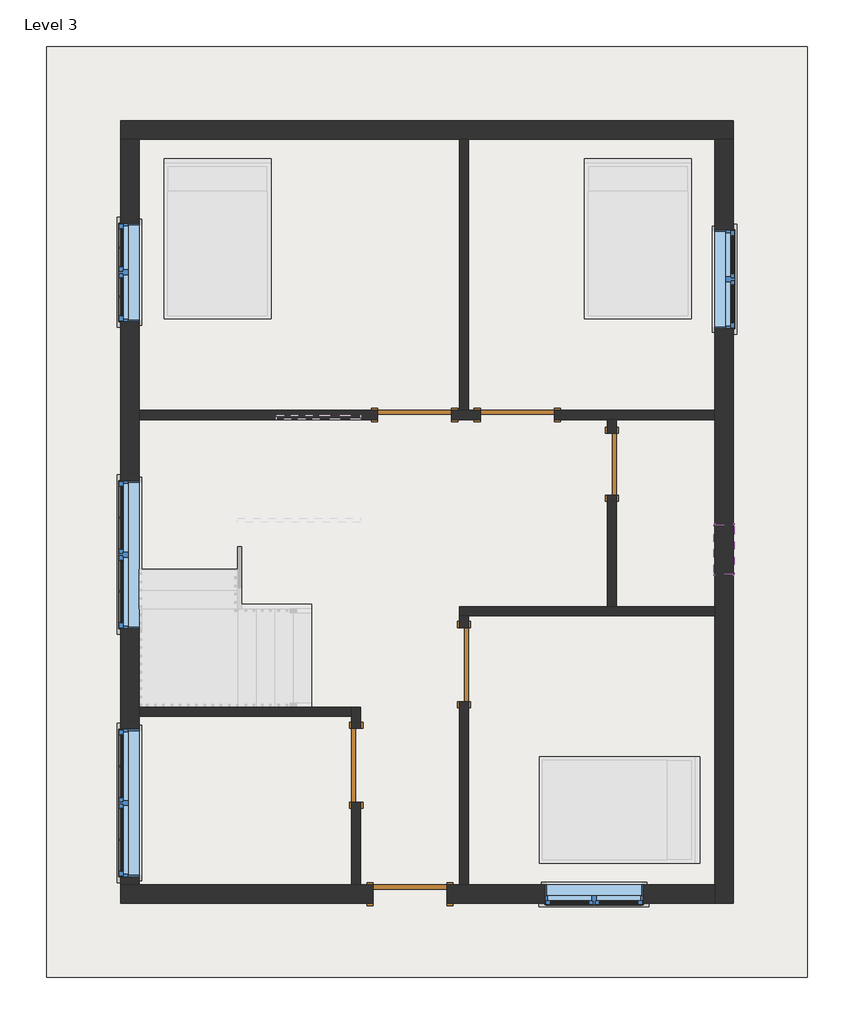
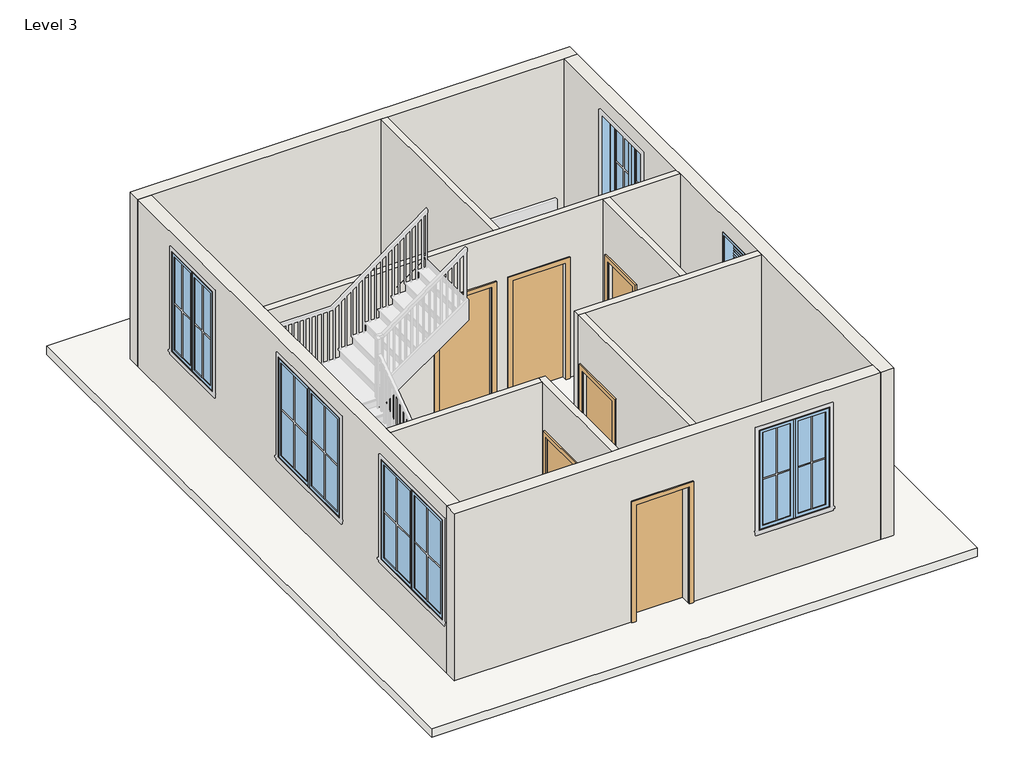
# One storey, part 1 of 3: 11 walls, 6 doors, 6 windows, 1 roof.
"""IFC4 building model written with IfcOpenShell, lengths in millimetres."""

from ifc_helpers import new_model, si_unit, frame, origin, place, context, project, spatial, polyline, outline, extrude, faceted_brep, transform, mapped, element, save
from components import door_f2b275c1, single_flush_door_3_e5f9f3c4, single_flush_door_3_305aa2a5, single_flush_door_3_a90ba1ad, window_casement_double_win_4_6ca1769e, window_casement_double_win_6_ce442eab, window_f2d8fef0

model = new_model("IFC4")

# Units and contexts
model_context = context("Model", 3, world=origin())
ifc_project = project(units=[si_unit("LENGTHUNIT", "METRE", prefix="MILLI")], contexts=[model_context])

# Site, building, storey
site = spatial("IfcSite", under=ifc_project)
building = spatial("IfcBuilding", under=site)
storey = spatial("IfcBuildingStorey", under=building, Name="Level 3", Elevation=6248.4)

# Doors
placement = place(None, origin())
door_shape = door_f2b275c1(model_context)
element("IfcDoor", 1, ObjectType="Single-Flush : 2'6\"", at=placement, inside=storey, context=model_context, shape_type="MappedRepresentation", body=[
    mapped(door_shape, transform((1031.6394609, 262.5126239, 6248.4), x_axis=(0.0, 1.0, 0.0), y_axis=(-1.0, 0.0, 0.0), z_axis=(0.0, 0.0, 1.0))),
])
single_flush_door_3_shape = single_flush_door_3_e5f9f3c4(model_context)
element("IfcDoor", 2, ObjectType="Single-Flush : door 3'", at=placement, inside=storey, context=model_context, shape_type="MappedRepresentation", body=[
    mapped(single_flush_door_3_shape, transform((-1406.7605391, 872.1126239, 6248.4), x_axis=(1.0, 0.0, 0.0), y_axis=(0.0, 1.0, 0.0), z_axis=(0.0, 0.0, 1.0))),
])
element("IfcDoor", 3, ObjectType="Single-Flush : door 3'", at=placement, inside=storey, context=model_context, shape_type="MappedRepresentation", body=[
    mapped(single_flush_door_3_shape, transform((-2130.6605391, -3458.5873761, 6248.4), x_axis=(0.0, 1.0, 0.0), y_axis=(-1.0, 0.0, 0.0), z_axis=(0.0, 0.0, 1.0))),
])
single_flush_door_3_2_shape = single_flush_door_3_305aa2a5(model_context)
element("IfcDoor", 4, ObjectType="Single-Flush : door 3'", at=placement, inside=storey, context=model_context, shape_type="MappedRepresentation", body=[
    mapped(single_flush_door_3_2_shape, transform((-136.7605391, 872.1126239, 6248.4), x_axis=(-1.0, 0.0, 0.0), y_axis=(0.0, -1.0, 0.0), z_axis=(0.0, 0.0, 1.0))),
])
element("IfcDoor", 5, ObjectType="Single-Flush : door 3'", at=placement, inside=storey, context=model_context, shape_type="MappedRepresentation", body=[
    mapped(single_flush_door_3_2_shape, transform((-797.1605391, -2213.9873761, 6248.4), x_axis=(0.0, 1.0, 0.0), y_axis=(-1.0, 0.0, 0.0), z_axis=(0.0, 0.0, 1.0))),
])
single_flush_door_3_3_shape = single_flush_door_3_a90ba1ad(model_context)
element("IfcDoor", 6, ObjectType="Single-Flush : door 3'", at=placement, inside=storey, context=model_context, shape_type="MappedRepresentation", body=[
    mapped(single_flush_door_3_3_shape, transform((-1463.9105391, -5052.4373761, 6248.4), x_axis=(-1.0, 0.0, 0.0), y_axis=(0.0, -1.0, 0.0), z_axis=(0.0, 0.0, 1.0))),
])

# Roof
element("IfcRoof", 7, ObjectType="Generic - 12\"", at=placement, inside=storey, context=model_context, shape_type="SweptSolid", body=[
    extrude(outline(polyline([(-5959.7105391, 5425.0626239), (3450.9894609, 5425.0626239), (3450.9894609, -6081.1373761), (-5959.7105391, -6081.1373761), (-5959.7105391, 5425.0626239)])), frame((0.0, 0.0, 6096.0), z_axis=(0.0, 0.0, 1.0), x_axis=(1.0, 0.0, 0.0)), (0.0, 0.0, 1.0), 152.4),
])

# Walls
element("IfcWall", 8, ObjectType="WALL 4.5\"", at=placement, inside=storey, context=model_context, shape_type="SweptSolid", body=[
    extrude(outline(polyline([(-854.3105391, 929.2626239), (-854.3105391, 4282.0626239), (-740.0105391, 4282.0626239), (-740.0105391, 929.2626239), (-854.3105391, 929.2626239)])), frame((0.0, 0.0, 6248.4), z_axis=(0.0, 0.0, 1.0), x_axis=(1.0, 0.0, 0.0)), (0.0, 0.0, 1.0), 3048.0),
])
element("IfcWall", 9, ObjectType="WALL 4.5\"", at=placement, inside=storey, context=model_context, shape_type="Brep", body=[
    faceted_brep([(-949.5605391, 814.9626239, 6248.4), (-593.9605391, 814.9626239, 6248.4), (-593.9605391, 814.9626239, 8382.0), (320.4394609, 814.9626239, 8382.0), (320.4394609, 814.9626239, 6248.4), (974.4894609, 814.9626239, 6248.4), (1088.7894609, 814.9626239, 6248.4), (2307.9894609, 814.9626239, 6248.4), (2307.9894609, 814.9626239, 9296.4), (1088.7894609, 814.9626239, 9296.4), (974.4894609, 814.9626239, 9296.4), (-4816.7105391, 814.9626239, 9296.4), (-4816.7105391, 814.9626239, 6248.4), (-1863.9605391, 814.9626239, 6248.4), (-1863.9605391, 814.9626239, 8382.0), (-949.5605391, 814.9626239, 8382.0), (-593.9605391, 929.2626239, 8382.0), (-593.9605391, 929.2626239, 6248.4), (-740.0105391, 929.2626239, 6248.4), (-854.3105391, 929.2626239, 6248.4), (-949.5605391, 929.2626239, 6248.4), (-949.5605391, 929.2626239, 8382.0), (-1863.9605391, 929.2626239, 8382.0), (-1863.9605391, 929.2626239, 6248.4), (-4816.7105391, 929.2626239, 6248.4), (-4816.7105391, 929.2626239, 9296.4), (-854.3105391, 929.2626239, 9296.4), (-740.0105391, 929.2626239, 9296.4), (2307.9894609, 929.2626239, 9296.4), (2307.9894609, 929.2626239, 6248.4), (320.4394609, 929.2626239, 6248.4), (320.4394609, 929.2626239, 8382.0)], [[[0, 1, 2, 3, 4, 5, 6, 7, 8, 9, 10, 11, 12, 13, 14, 15]], [[16, 17, 18, 19, 20, 21, 22, 23, 24, 25, 26, 27, 28, 29, 30, 31]], [[13, 12, 24, 23]], [[30, 29, 7, 6, 5, 4]], [[20, 19, 18, 17, 1, 0]], [[8, 7, 29, 28]], [[12, 11, 25, 24]], [[21, 20, 0, 15]], [[22, 21, 15, 14]], [[23, 22, 14, 13]], [[2, 1, 17, 16]], [[3, 2, 16, 31]], [[4, 3, 31, 30]], [[11, 10, 9, 8, 28, 27, 26, 25]]]),
])
element("IfcWall", 10, ObjectType="WALL 4.5\"", at=placement, inside=storey, context=model_context, shape_type="SweptSolid", body=[
    extrude(outline(polyline([(814.9626239, 6248.4), (643.5126239, 6248.4), (643.5126239, 8280.4), (-118.4873761, 8280.4), (-118.4873761, 6248.4), (-1496.4373761, 6248.4), (-1496.4373761, 9296.4), (814.9626239, 9296.4), (814.9626239, 6248.4)])), frame((974.4894609, 0.0, 0.0), z_axis=(1.0, 0.0, 0.0), x_axis=(0.0, 1.0, 0.0)), (0.0, 0.0, 1.0), 114.3),
])
element("IfcWall", 11, ObjectType="WALL 4.5\"", at=placement, inside=storey, context=model_context, shape_type="Brep", body=[
    faceted_brep([(2307.9894609, -1496.4373761, 6248.4), (1088.7894609, -1496.4373761, 6248.4), (974.4894609, -1496.4373761, 6248.4), (-854.3105391, -1496.4373761, 6248.4), (-854.3105391, -1496.4373761, 9296.4), (974.4894609, -1496.4373761, 9296.4), (1088.7894609, -1496.4373761, 9296.4), (2307.9894609, -1496.4373761, 9296.4), (2307.9894609, -1610.7373761, 6248.4), (2307.9894609, -1610.7373761, 9296.4), (-740.0105391, -1610.7373761, 9296.4), (-854.3105391, -1610.7373761, 9296.4), (-854.3105391, -1610.7373761, 6248.4), (-740.0105391, -1610.7373761, 6248.4)], [[[0, 1, 2, 3, 4, 5, 6, 7]], [[8, 9, 10, 11, 12, 13]], [[3, 2, 1, 0, 8, 13, 12]], [[0, 7, 9, 8]], [[4, 3, 12, 11]], [[7, 6, 5, 4, 11, 10, 9]]]),
])
element("IfcWall", 12, ObjectType="WALL 4.5\"", at=placement, inside=storey, context=model_context, shape_type="SweptSolid", body=[
    extrude(outline(polyline([(-1610.7373761, 6248.4), (-1756.7873761, 6248.4), (-1756.7873761, 8382.0), (-2671.1873761, 8382.0), (-2671.1873761, 6248.4), (-4938.1373761, 6248.4), (-4938.1373761, 9296.4), (-1610.7373761, 9296.4), (-1610.7373761, 6248.4)])), frame((-854.3105391, 0.0, 0.0), z_axis=(1.0, 0.0, 0.0), x_axis=(0.0, 1.0, 0.0)), (0.0, 0.0, 1.0), 114.3),
])
element("IfcWall", 13, ObjectType="WALL 4.5\"", at=placement, inside=storey, context=model_context, shape_type="Brep", body=[
    faceted_brep([(-2073.5105391, -3001.3873761, 8382.0), (-2073.5105391, -3001.3873761, 6248.4), (-2073.5105391, -2741.0373761, 6248.4), (-2073.5105391, -2741.0373761, 9296.4), (-2073.5105391, -4938.1373761, 9296.4), (-2073.5105391, -4938.1373761, 6248.4), (-2073.5105391, -3915.7873761, 6248.4), (-2073.5105391, -3915.7873761, 8382.0), (-2187.8105391, -2741.0373761, 6248.4), (-2187.8105391, -2855.3373761, 6248.4), (-2187.8105391, -3001.3873761, 6248.4), (-2187.8105391, -3001.3873761, 8382.0), (-2187.8105391, -3915.7873761, 8382.0), (-2187.8105391, -3915.7873761, 6248.4), (-2187.8105391, -4938.1373761, 6248.4), (-2187.8105391, -4938.1373761, 9296.4), (-2187.8105391, -2855.3373761, 9296.4), (-2187.8105391, -2741.0373761, 9296.4)], [[[0, 1, 2, 3, 4, 5, 6, 7]], [[8, 9, 10, 11, 12, 13, 14, 15, 16, 17]], [[6, 5, 14, 13]], [[2, 1, 10, 9, 8]], [[5, 4, 15, 14]], [[3, 2, 8, 17]], [[11, 10, 1, 0]], [[12, 11, 0, 7]], [[13, 12, 7, 6]], [[4, 3, 17, 16, 15]]]),
])
element("IfcWall", 14, ObjectType="WALL 4.5\"", at=placement, inside=storey, context=model_context, shape_type="SweptSolid", body=[
    extrude(outline(polyline([(-4816.7105391, -2741.0373761), (-2187.8105391, -2741.0373761), (-2187.8105391, -2855.3373761), (-4816.7105391, -2855.3373761), (-4816.7105391, -2741.0373761)])), frame((0.0, 0.0, 6248.4), z_axis=(0.0, 0.0, 1.0), x_axis=(1.0, 0.0, 0.0)), (0.0, 0.0, 1.0), 3048.0),
])
element("IfcWall", 15, ObjectType="WALL 9\"", at=placement, inside=storey, context=model_context, shape_type="Brep", body=[
    faceted_brep([(-5045.3105391, 4282.0626239, 6248.4), (-4816.7105391, 4282.0626239, 6248.4), (-854.3105391, 4282.0626239, 6248.4), (-740.0105391, 4282.0626239, 6248.4), (2307.9894609, 4282.0626239, 6248.4), (2536.5894609, 4282.0626239, 6248.4), (2536.5894609, 4282.0626239, 9296.4), (2307.9894609, 4282.0626239, 9296.4), (-740.0105391, 4282.0626239, 9296.4), (-854.3105391, 4282.0626239, 9296.4), (-4816.7105391, 4282.0626239, 9296.4), (-5045.3105391, 4282.0626239, 9296.4), (-5045.3105391, 4510.6626239, 6248.4), (-5045.3105391, 4510.6626239, 9296.4), (2536.5894609, 4510.6626239, 9296.4), (2536.5894609, 4510.6626239, 6248.4)], [[[0, 1, 2, 3, 4, 5, 6, 7, 8, 9, 10, 11]], [[12, 13, 14, 15]], [[5, 4, 3, 2, 1, 0, 12, 15]], [[6, 5, 15, 14]], [[0, 11, 13, 12]], [[11, 10, 9, 8, 7, 6, 14, 13]]]),
])
element("IfcWall", 16, ObjectType="WALL 9\"", at=placement, inside=storey, context=model_context, shape_type="Brep", body=[
    faceted_brep([(2307.9894609, 4282.0626239, 6248.4), (2307.9894609, 929.2626239, 6248.4), (2307.9894609, 814.9626239, 6248.4), (2307.9894609, -1496.4373761, 6248.4), (2307.9894609, -1610.7373761, 6248.4), (2307.9894609, -4938.1373761, 6248.4), (2307.9894609, -5166.7373761, 6248.4), (2307.9894609, -5166.7373761, 9296.4), (2307.9894609, -4938.1373761, 9296.4), (2307.9894609, -1610.7373761, 9296.4), (2307.9894609, -1496.4373761, 9296.4), (2307.9894609, 814.9626239, 9296.4), (2307.9894609, 929.2626239, 9296.4), (2307.9894609, 4282.0626239, 9296.4), (2307.9894609, 1938.9126239, 8991.6), (2307.9894609, 1938.9126239, 7162.8), (2307.9894609, 3158.1126239, 7162.8), (2307.9894609, 3158.1126239, 8991.6), (2307.9894609, -486.7873761, 8991.6), (2307.9894609, -1096.3873761, 8991.6), (2307.9894609, -1096.3873761, 8382.0), (2307.9894609, -486.7873761, 8382.0), (2536.5894609, 4282.0626239, 6248.4), (2536.5894609, 4282.0626239, 9296.4), (2536.5894609, -5166.7373761, 9296.4), (2536.5894609, -5166.7373761, 6248.4), (2536.5894609, 1938.9126239, 8991.6), (2536.5894609, 3158.1126239, 8991.6), (2536.5894609, 3158.1126239, 7162.8), (2536.5894609, 1938.9126239, 7162.8), (2536.5894609, -486.7873761, 8991.6), (2536.5894609, -486.7873761, 8382.0), (2536.5894609, -1096.3873761, 8382.0), (2536.5894609, -1096.3873761, 8991.6)], [[[0, 1, 2, 3, 4, 5, 6, 7, 8, 9, 10, 11, 12, 13], [14, 15, 16, 17], [18, 19, 20, 21]], [[22, 23, 24, 25], [26, 27, 28, 29], [30, 31, 32, 33]], [[6, 5, 4, 3, 2, 1, 0, 22, 25]], [[0, 13, 23, 22]], [[7, 6, 25, 24]], [[15, 14, 26, 29]], [[16, 15, 29, 28]], [[17, 16, 28, 27]], [[14, 17, 27, 26]], [[31, 30, 18, 21]], [[32, 31, 21, 20]], [[33, 32, 20, 19]], [[30, 33, 19, 18]], [[13, 12, 11, 10, 9, 8, 7, 24, 23]]]),
])
element("IfcWall", 17, ObjectType="WALL 9\"", at=placement, inside=storey, context=model_context, shape_type="Brep", body=[
    faceted_brep([(-1921.1105391, -4938.1373761, 8382.0), (-1921.1105391, -4938.1373761, 6248.4), (-2073.5105391, -4938.1373761, 6248.4), (-2187.8105391, -4938.1373761, 6248.4), (-4816.7105391, -4938.1373761, 6248.4), (-5045.3105391, -4938.1373761, 6248.4), (-5045.3105391, -4938.1373761, 9296.4), (-4816.7105391, -4938.1373761, 9296.4), (-2187.8105391, -4938.1373761, 9296.4), (-2073.5105391, -4938.1373761, 9296.4), (-854.3105391, -4938.1373761, 9296.4), (-740.0105391, -4938.1373761, 9296.4), (2307.9894609, -4938.1373761, 9296.4), (2307.9894609, -4938.1373761, 6248.4), (-740.0105391, -4938.1373761, 6248.4), (-854.3105391, -4938.1373761, 6248.4), (-1006.7105391, -4938.1373761, 6248.4), (-1006.7105391, -4938.1373761, 8382.0), (202.9644609, -4938.1373761, 8991.6), (202.9644609, -4938.1373761, 7162.8), (1422.1644609, -4938.1373761, 7162.8), (1422.1644609, -4938.1373761, 8991.6), (-5045.3105391, -5166.7373761, 6248.4), (-1921.1105391, -5166.7373761, 6248.4), (-1921.1105391, -5166.7373761, 8382.0), (-1006.7105391, -5166.7373761, 8382.0), (-1006.7105391, -5166.7373761, 6248.4), (2307.9894609, -5166.7373761, 6248.4), (2307.9894609, -5166.7373761, 9296.4), (-5045.3105391, -5166.7373761, 9296.4), (202.9644609, -5166.7373761, 8991.6), (1422.1644609, -5166.7373761, 8991.6), (1422.1644609, -5166.7373761, 7162.8), (202.9644609, -5166.7373761, 7162.8)], [[[0, 1, 2, 3, 4, 5, 6, 7, 8, 9, 10, 11, 12, 13, 14, 15, 16, 17], [18, 19, 20, 21]], [[22, 23, 24, 25, 26, 27, 28, 29], [30, 31, 32, 33]], [[5, 4, 3, 2, 1, 23, 22]], [[16, 15, 14, 13, 27, 26]], [[13, 12, 28, 27]], [[6, 5, 22, 29]], [[19, 18, 30, 33]], [[20, 19, 33, 32]], [[21, 20, 32, 31]], [[18, 21, 31, 30]], [[24, 23, 1, 0]], [[25, 24, 0, 17]], [[26, 25, 17, 16]], [[12, 11, 10, 9, 8, 7, 6, 29, 28]]]),
])
element("IfcWall", 18, ObjectType="WALL 9\"", at=placement, inside=storey, context=model_context, shape_type="Brep", body=[
    faceted_brep([(-4816.7105391, -4938.1373761, 6248.4), (-4816.7105391, -2855.3373761, 6248.4), (-4816.7105391, -2741.0373761, 6248.4), (-4816.7105391, 814.9626239, 6248.4), (-4816.7105391, 929.2626239, 6248.4), (-4816.7105391, 4282.0626239, 6248.4), (-4816.7105391, 4282.0626239, 9296.4), (-4816.7105391, 929.2626239, 9296.4), (-4816.7105391, 814.9626239, 9296.4), (-4816.7105391, -2741.0373761, 9296.4), (-4816.7105391, -2855.3373761, 9296.4), (-4816.7105391, -4938.1373761, 9296.4), (-4816.7105391, -3010.9123761, 8991.6), (-4816.7105391, -3010.9123761, 7162.8), (-4816.7105391, -4839.7123761, 7162.8), (-4816.7105391, -4839.7123761, 8991.6), (-4816.7105391, 59.3126239, 8991.6), (-4816.7105391, 59.3126239, 7162.8), (-4816.7105391, -1769.4873761, 7162.8), (-4816.7105391, -1769.4873761, 8991.6), (-4816.7105391, 3243.8376239, 8991.6), (-4816.7105391, 3243.8376239, 7162.8), (-4816.7105391, 2024.6376239, 7162.8), (-4816.7105391, 2024.6376239, 8991.6), (-5045.3105391, -4938.1373761, 6248.4), (-5045.3105391, -4938.1373761, 9296.4), (-5045.3105391, 4282.0626239, 9296.4), (-5045.3105391, 4282.0626239, 6248.4), (-5045.3105391, -3010.9123761, 8991.6), (-5045.3105391, -4839.7123761, 8991.6), (-5045.3105391, -4839.7123761, 7162.8), (-5045.3105391, -3010.9123761, 7162.8), (-5045.3105391, 59.3126239, 8991.6), (-5045.3105391, -1769.4873761, 8991.6), (-5045.3105391, -1769.4873761, 7162.8), (-5045.3105391, 59.3126239, 7162.8), (-5045.3105391, 3243.8376239, 8991.6), (-5045.3105391, 2024.6376239, 8991.6), (-5045.3105391, 2024.6376239, 7162.8), (-5045.3105391, 3243.8376239, 7162.8)], [[[0, 1, 2, 3, 4, 5, 6, 7, 8, 9, 10, 11], [12, 13, 14, 15], [16, 17, 18, 19], [20, 21, 22, 23]], [[24, 25, 26, 27], [28, 29, 30, 31], [32, 33, 34, 35], [36, 37, 38, 39]], [[5, 4, 3, 2, 1, 0, 24, 27]], [[6, 5, 27, 26]], [[0, 11, 25, 24]], [[13, 12, 28, 31]], [[14, 13, 31, 30]], [[15, 14, 30, 29]], [[12, 15, 29, 28]], [[17, 16, 32, 35]], [[18, 17, 35, 34]], [[19, 18, 34, 33]], [[16, 19, 33, 32]], [[21, 20, 36, 39]], [[22, 21, 39, 38]], [[23, 22, 38, 37]], [[20, 23, 37, 36]], [[11, 10, 9, 8, 7, 6, 26, 25]]]),
])

# Windows
window_casement_double_win_4_shape = window_casement_double_win_4_6ca1769e(model_context)
element("IfcWindow", 19, ObjectType="Window-Casement-Double : win 4'", at=placement, inside=storey, context=model_context, shape_type="MappedRepresentation", body=[
    mapped(window_casement_double_win_4_shape, transform((812.5644609, -5052.4373761, 6248.4), x_axis=(-1.0, 0.0, 0.0), y_axis=(0.0, -1.0, 0.0), z_axis=(0.0, 0.0, 1.0))),
])
element("IfcWindow", 20, ObjectType="Window-Casement-Double : win 4'", at=placement, inside=storey, context=model_context, shape_type="MappedRepresentation", body=[
    mapped(window_casement_double_win_4_shape, transform((2422.2894609, 2548.5126239, 6248.4), x_axis=(0.0, -1.0, 0.0), y_axis=(1.0, 0.0, 0.0), z_axis=(0.0, 0.0, 1.0))),
])
element("IfcWindow", 21, ObjectType="Window-Casement-Double : win 4'", at=placement, inside=storey, context=model_context, shape_type="MappedRepresentation", body=[
    mapped(window_casement_double_win_4_shape, transform((-4931.0105391, 2634.2376239, 6248.4), x_axis=(0.0, 1.0, 0.0), y_axis=(-1.0, 0.0, 0.0), z_axis=(0.0, 0.0, 1.0))),
])
window_casement_double_win_6_shape = window_casement_double_win_6_ce442eab(model_context)
element("IfcWindow", 22, ObjectType="Window-Casement-Double : win 6'", at=placement, inside=storey, context=model_context, shape_type="MappedRepresentation", body=[
    mapped(window_casement_double_win_6_shape, transform((-4931.0105391, -3925.3123761, 6248.4), x_axis=(0.0, 1.0, 0.0), y_axis=(-1.0, 0.0, 0.0), z_axis=(0.0, 0.0, 1.0))),
])
element("IfcWindow", 23, ObjectType="Window-Casement-Double : win 6'", at=placement, inside=storey, context=model_context, shape_type="MappedRepresentation", body=[
    mapped(window_casement_double_win_6_shape, transform((-4931.0105391, -855.0873761, 6248.4), x_axis=(0.0, 1.0, 0.0), y_axis=(-1.0, 0.0, 0.0), z_axis=(0.0, 0.0, 1.0))),
])
window_shape = window_f2d8fef0(model_context)
element("IfcWindow", 24, ObjectType="Window-Louvers : 24\" x 24\"", at=placement, inside=storey, context=model_context, shape_type="MappedRepresentation", body=[
    mapped(window_shape, transform((2428.6394609, -791.5873761, 7467.6), x_axis=(0.0, -1.0, 0.0), y_axis=(1.0, 0.0, 0.0), z_axis=(0.0, 0.0, 1.0))),
])

save(model, "model.ifc")

# Revit data of these elements
# Type "Single-Flush : 2'6\""
#   Type Mark = "9"
#   Construction Type Id = "MDOOR"
#   Assembly Code = "C1020"
#   Analytic Construction = "Metal"
#   Thickness = 0' - 2"
#   Heat Transfer Coefficient (U) = 0.651978 BTU/(h·ft²·°F)
#   Height = 6' - 8"
#   Trim Projection Ext = 0' - 1"
#   Trim Projection Int = 0' - 1"
#   Trim Width = 0' - 3"
#   Width = 2' - 6"
#   Define Thermal Properties by = 1
#   Door Material = Door - Panel
#   Frame Material = Door - Frame
#   Visual Light Transmittance = 0
#   Solar Heat Gain Coefficient = 0
#   Function = (empty or 0)
#   Wall Closure = (empty or 0)
# Type "Single-Flush : door 3'"
#   Type Mark = "8"
#   Construction Type Id = "MDOOR"
#   Assembly Code = "C1020"
#   Analytic Construction = "Metal"
#   Thickness = 0' - 2"
#   Heat Transfer Coefficient (U) = 0.651978 BTU/(h·ft²·°F)
#   Height = 7' - 0"
#   Trim Projection Ext = 0' - 1"
#   Trim Projection Int = 0' - 1"
#   Trim Width = 0' - 3"
#   Width = 3' - 0"
#   Define Thermal Properties by = 1
#   Door Material = Door - Panel
#   Frame Material = Door - Frame
#   Visual Light Transmittance = 0
#   Solar Heat Gain Coefficient = 0
#   Function = (empty or 0)
#   Wall Closure = (empty or 0)
# Type "Generic - 12\""
#   Assembly Code = "B1020"
#   Layers, outside or top first: 0' - 6" no material (function 1)
# Type "WALL 4.5\""
#   Assembly Code = "B2010"
#   Layers, outside or top first: 0' - 4 1/2" no material (function 1)
# Type "WALL 9\""
#   Assembly Code = "B2010"
#   Layers, outside or top first: 0' - 9" no material (function 1)
# Type "Window-Casement-Double : win 4'"
#   Type Mark = "19"
#   Fire Rating = "0.5h"
#   Assembly Code = "B2020100"
#   Analytic Construction = "Double glazing - domestic"
#   Frame Extension [instance default] = 0' - 0 1/4"
#   Window Inset [instance default] = 0' - 0"
#   Wall Thickness [instance default] = 0' - 6"
#   Interior Wall Closure [instance default] = 0' - 2 1/4"
#   Half Width = 2' - 0"
#   Visual Light Transmittance = 0.81
#   Thermal Resistance (R) = 1.8146 (h·ft²·°F)/BTU
#   Solar Heat Gain Coefficient = 0.76
#   Rough Width = 4' - 0 1/2"
#   Rough Height = 6' - 0 1/2"
#   Height = 6' - 0"
#   Heat Transfer Coefficient (U) = 0.5511 BTU/(h·ft²·°F)
#   Exterior Wall Closure [instance default] = 0' - 1 1/4"
#   Extension Jamb [instance default] = 0' - 2 1/4"
#   Default Sill Height = 3' - 0"
#   Width = 4' - 0"
#   Muntin Visibility = yes
#   Interior Trim Visibility [instance default] = yes
#   Exterior Trim Visibility [instance default] = yes
#   Extension Jamb Visibility [instance default] = yes
#   Interior Trim Material = Wood - Stained
#   Muntin Pattern = Muntin Pattern_2x2 : Muntin Pattern_2x2
#   Interior Trim = Trim-Window-Interior-Flat : Picture Frame
#   Interior Frame Material = Wood - Stained
#   Glass Panel Material = Glass
#   Exterior Trim Material = Clad - White
#   Exterior Trim = Trim-Window-Exterior-Flat : with Sill
#   Exterior Frame Material = Clad - White
#   Wall Closure = (empty or 0)
# Type "Window-Casement-Double : win 6'"
#   Type Mark = "18"
#   Fire Rating = "0.5h"
#   Assembly Code = "B2020100"
#   Analytic Construction = "Double glazing - domestic"
#   Frame Extension [instance default] = 0' - 0 1/4"
#   Window Inset [instance default] = 0' - 0"
#   Wall Thickness [instance default] = 0' - 6"
#   Interior Wall Closure [instance default] = 0' - 2 1/4"
#   Half Width = 3' - 0"
#   Visual Light Transmittance = 0.81
#   Thermal Resistance (R) = 1.8146 (h·ft²·°F)/BTU
#   Solar Heat Gain Coefficient = 0.76
#   Rough Width = 6' - 0 1/2"
#   Rough Height = 6' - 0 1/2"
#   Height = 6' - 0"
#   Heat Transfer Coefficient (U) = 0.5511 BTU/(h·ft²·°F)
#   Exterior Wall Closure [instance default] = 0' - 1 1/4"
#   Extension Jamb [instance default] = 0' - 2 1/4"
#   Default Sill Height = 3' - 0"
#   Width = 6' - 0"
#   Muntin Visibility = yes
#   Interior Trim Visibility [instance default] = yes
#   Exterior Trim Visibility [instance default] = yes
#   Extension Jamb Visibility [instance default] = yes
#   Interior Trim Material = Wood - Stained
#   Muntin Pattern = Muntin Pattern_2x2 : Muntin Pattern_2x2
#   Interior Trim = Trim-Window-Interior-Flat : Picture Frame
#   Interior Frame Material = Wood - Stained
#   Glass Panel Material = Glass
#   Exterior Trim Material = Clad - White
#   Exterior Trim = Trim-Window-Exterior-Flat : with Sill
#   Exterior Frame Material = Clad - White
#   Wall Closure = (empty or 0)
# Type "Window-Louvers : 24\" x 24\""
#   Type Mark = "20"
#   Construction Type Id = "GSP4R"
#   Assembly Code = "B20"
#   Analytic Construction = "1/8 in Pilkington single glazing"
#   Visual Light Transmittance = 0.9
#   Thermal Resistance (R) = 1.53941 (h·ft²·°F)/BTU
#   Solar Heat Gain Coefficient = 0.78
#   Max Height = 1' - 11.74264"
#   Height = 2' - 0"
#   Heat Transfer Coefficient (U) = 0.6496 BTU/(h·ft²·°F)
#   Blade Width [instance default] = 1' - 10 1/2"
#   Blade Vertical Thickness = 0' - 0.35355"
#   Blade Thickness = 0' - 0 1/4"
#   Blade Spacing = 0' - 1 1/2"
#   Blade Height = 0' - 1.85355"
#   Blade Depth = 0' - 3"
#   Blade Angle = 45.00°
#   Default Sill Height = 3' - 0"
#   Trim Projection_Exterior = 0' - 0 1/2"
#   Trim Projection_Interior = 0' - 0 1/2"
#   Trim Width_Exterior = 0' - 1 1/2"
#   Trim Width_Interior = 0' - 1 1/2"
#   Width = 2' - 0"
#   Max Blade Count = 12
#   Define Thermal Properties by = 1
#   Blade Count = 12
#   Frame Material = Birch
#   Louver Material = Birch
#   Trim Exterior Material = Birch
#   Trim Interior Material = Birch
#   Wall Closure = (empty or 0)
# Element 1 (IfcDoor, "Single-Flush : 2'6\"")
#   Phase Created = New Construction
#   Materials on its faces: "Door - Frame", "Door - Panel"
# Elements 2, 3, 4, 5, 6 (IfcDoor, "Single-Flush : door 3'")
#   Phase Created = New Construction
#   Materials on its faces: "Door - Frame", "Door - Panel"
# Element 7 (IfcRoof, "Generic - 12\"")
#   built-in parameter 1001705 = 20.5 (stored number, unit not read)
#   built-in parameter 1001701 = -0.5 (stored number, unit not read)
#   built-in parameter 1001710 = 33615
#   Phase Created = New Construction
#   Materials on its faces: "Wood Planks", "Wood - Stained"
# Elements 8, 9, 10, 11, 12, 13, 14 (IfcWall, "WALL 4.5\"")
#   Top Offset = 0' - 0"
#   Base Offset = 0' - 0"
#   Unconnected Height = 10' - 0"
#   wall height = 10' - 0"
#   Phase Created = New Construction
#   Base Constraint = Level 3
#   Materials on its faces: "Default Wall"
# Elements 15, 16, 17, 18 (IfcWall, "WALL 9\"")
#   Top Offset = 0' - 0"
#   Base Offset = 0' - 0"
#   Unconnected Height = 10' - 0"
#   wall height = 10' - 0"
#   Phase Created = New Construction
#   Base Constraint = Level 3
#   Materials on its faces: "Default Wall", "Door - Frame"
# Element 19 (IfcWindow, "Window-Casement-Double : win 4'")
#   Mark = "15"
#   Window Inset = 0' - 0"
#   Interior Wall Closure = 0' - 2 1/4"
#   Frame Extension = 0' - 0 1/4"
#   Exterior Wall Closure = 0' - 1 1/4"
#   Interior Trim Visibility = yes
#   Exterior Trim Visibility = yes
#   Phase Created = New Construction
#   Materials on its faces: "Wood - Stained", "Glass", "Clad - White"
# Element 20 (IfcWindow, "Window-Casement-Double : win 4'")
#   Mark = "16"
#   Window Inset = 0' - 0"
#   Interior Wall Closure = 0' - 2 1/4"
#   Frame Extension = 0' - 0 1/4"
#   Exterior Wall Closure = 0' - 1 1/4"
#   Interior Trim Visibility = yes
#   Exterior Trim Visibility = yes
#   Phase Created = New Construction
#   Materials on its faces: "Wood - Stained", "Glass", "Clad - White"
# Element 21 (IfcWindow, "Window-Casement-Double : win 4'")
#   Mark = "17"
#   Window Inset = 0' - 0"
#   Interior Wall Closure = 0' - 2 1/4"
#   Frame Extension = 0' - 0 1/4"
#   Exterior Wall Closure = 0' - 1 1/4"
#   Interior Trim Visibility = yes
#   Exterior Trim Visibility = yes
#   Phase Created = New Construction
#   Materials on its faces: "Wood - Stained", "Glass", "Clad - White"
# Element 22 (IfcWindow, "Window-Casement-Double : win 6'")
#   Mark = "13"
#   Window Inset = 0' - 0"
#   Interior Wall Closure = 0' - 2 1/4"
#   Frame Extension = 0' - 0 1/4"
#   Exterior Wall Closure = 0' - 1 1/4"
#   Interior Trim Visibility = yes
#   Exterior Trim Visibility = yes
#   Phase Created = New Construction
#   Materials on its faces: "Wood - Stained", "Glass", "Clad - White"
# Element 23 (IfcWindow, "Window-Casement-Double : win 6'")
#   Mark = "14"
#   Window Inset = 0' - 0"
#   Interior Wall Closure = 0' - 2 1/4"
#   Frame Extension = 0' - 0 1/4"
#   Exterior Wall Closure = 0' - 1 1/4"
#   Interior Trim Visibility = yes
#   Exterior Trim Visibility = yes
#   Phase Created = New Construction
#   Materials on its faces: "Wood - Stained", "Glass", "Clad - White"
# Element 24 (IfcWindow, "Window-Louvers : 24\" x 24\"")
#   Mark = "18"
#   Blade Width = 1' - 10 1/2"
#   Phase Created = New Construction
#   Materials on its faces: "Birch"
# Materials
#   "Door - Panel": class "Wood", colour RGB 210 159 95, transparency 0, Cost = 0
#   "Door - Frame": colour RGB 118 70 51, transparency 0, Cost = 0
#   "Wood - Stained": class "Wood", colour RGB 224 178 126, transparency 0, Cost = 0
#   "Glass": class "Glass", colour RGB 0 128 192, transparency 0.75, Description = "Soda Lime Glass", Cost = 0
#   "Clad - White": class "Wood", colour RGB 242 242 238, transparency 0, Cost = 0
#   "Birch": class "Wood", colour RGB 224 178 126, transparency 0, Description = "Betula Alleghaniensis", Cost = 0
#   "Wood Planks": class "Wood", colour RGB 193 160 115, transparency 0, Description = "Physical material.", Cost = 0
#   "Default Wall": colour RGB 128 128 128, transparency 0, Cost = 0
